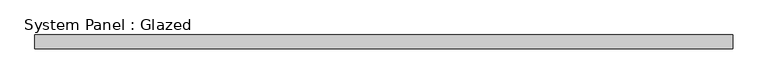
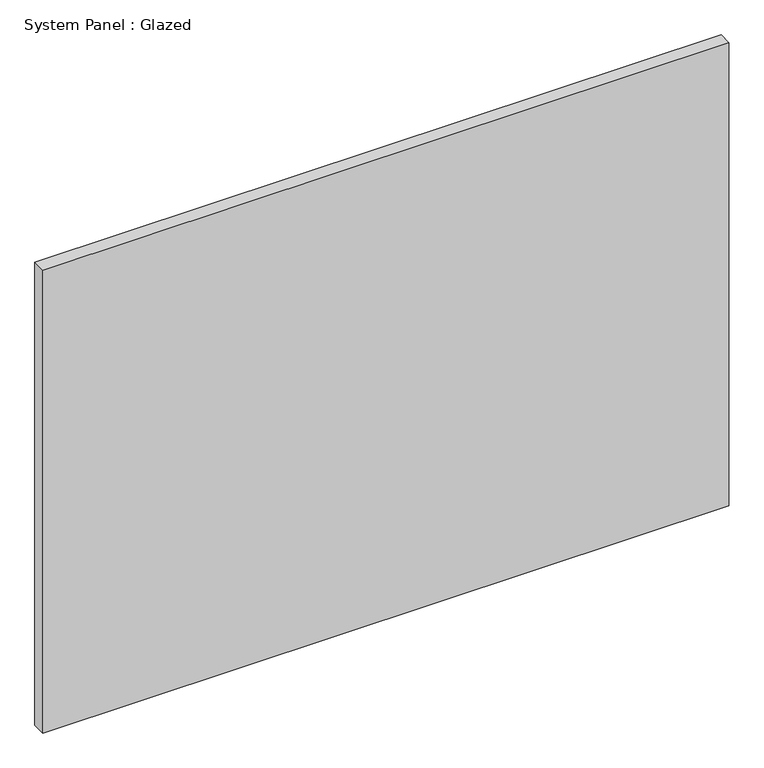
"""IFC4 building model written with IfcOpenShell, lengths in millimetres: plate geometry, System Panel : Glazed."""

from ifc_helpers import new_model, si_unit, origin, origin_with_axes, place, context, project, spatial, polyline, outline, extrude, source, transform, mapped, element, save


def system_panel_glazed_6a79ef8b(model_context):
    return source(origin(), model_context, "Body", "SweptSolid", [
        extrude(outline(polyline([(633.9416667, 19.05), (-633.9416667, 19.05), (-633.9416667, 44.45), (633.9416667, 44.45), (633.9416667, 19.05)])), origin_with_axes(), (0.0, 0.0, 1.0), 904.7272807),
    ])


if __name__ == "__main__":
    model = new_model("IFC4")
    model_context = context("Model", 3, world=origin())
    ifc_project = project(units=[si_unit("LENGTHUNIT", "METRE", prefix="MILLI")], contexts=[model_context])
    site = spatial("IfcSite", under=ifc_project)
    building = spatial("IfcBuilding", under=site)
    placement = place(None, origin())
    system_panel_glazed_shape = system_panel_glazed_6a79ef8b(model_context)
    element("IfcPlate", 1, ObjectType="System Panel : Glazed", at=placement, inside=building, context=model_context, shape_type="MappedRepresentation", body=[
        mapped(system_panel_glazed_shape, transform((0.0, 0.0, 0.0), x_axis=(1.0, 0.0, 0.0), y_axis=(0.0, 1.0, 0.0), z_axis=(0.0, 0.0, 1.0))),
    ])
    save(model, "model.ifc")

# Revit data of these elements
# Type "System Panel : Glazed"
#   Construction Type Id = "GSP4R"
#   Analytic Construction = "1/8 in Pilkington single glazing"
#   Visual Light Transmittance = 0.9
#   Solar Heat Gain Coefficient = 0.86
#   Heat Transfer Coefficient (U) = 1.18115 BTU/(h·ft²·°F)
#   Define Thermal Properties by = 1
# Element 1 (IfcPlate, "System Panel : Glazed")
#   Materials on its faces: "Glass"
# Materials
#   "Glass": class "Glass", colour RGB 0 128 192, transparency 0.75, Description = "Soda Lime Glass", Cost = 0
